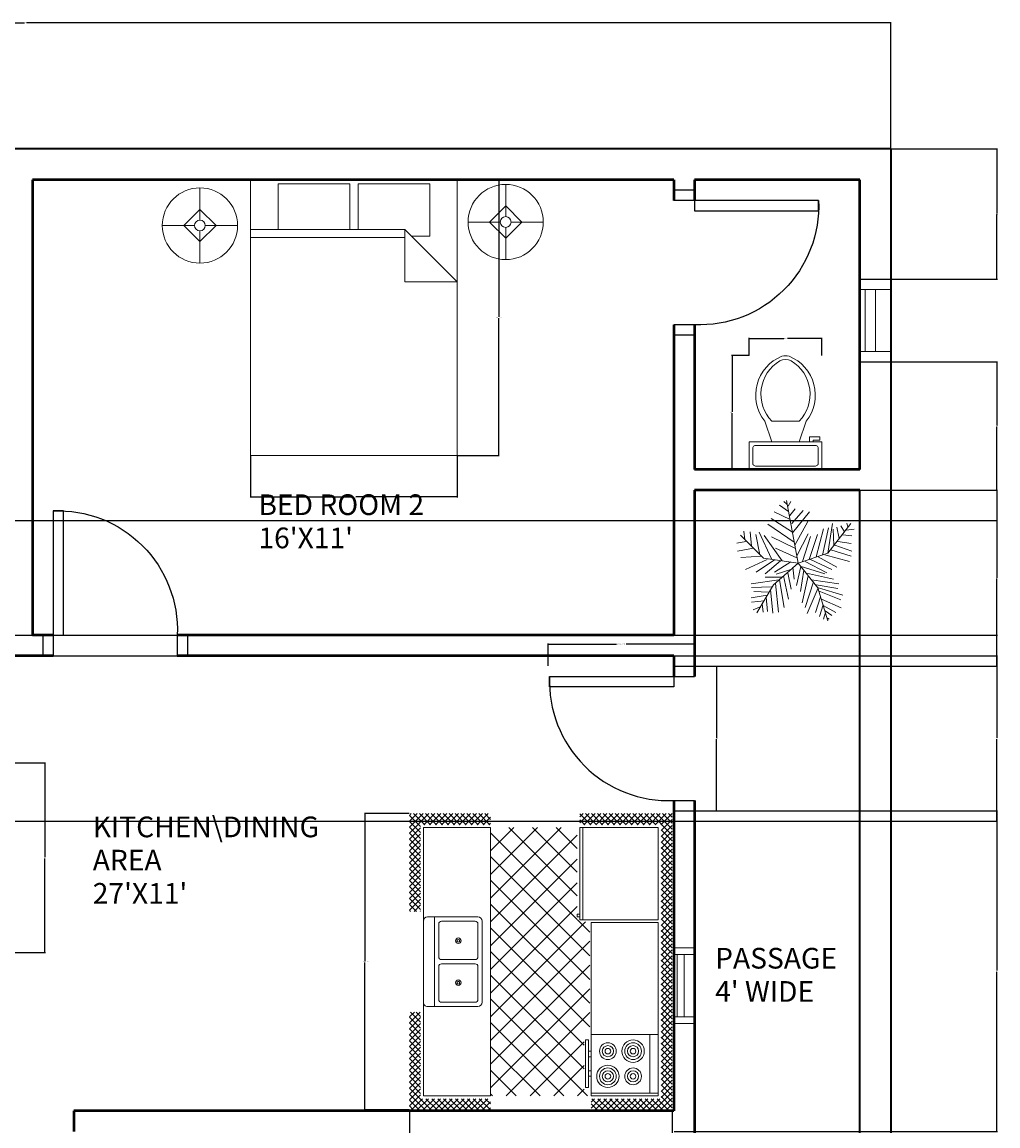
# Model space of a CAD drawing. Units: inches. Extents: x 156 to 720, y 11 to 679.
# Tile 5 of 5: x 437 to 720, y 359 to 679. Entities that reach past the tile are written whole.
import ezdxf

# ---------------------------------------------------------------- set-up
doc = ezdxf.new("R2010")
doc.units = ezdxf.units.IN
for name, color, linetype, lineweight in [('A-ANNO-DIMS', 2, 'Continuous', 18), ('A-AREA-IDEN', 7, 'Continuous', 25), ('A-DOOR', 3, 'Continuous', 25), ('A-FLOR-FIXT', 9, 'Continuous', 18), ('A-FURN', 8, 'Continuous', 18), ('A-GLAZ', 4, 'Continuous', 18), ('A-WALL', 7, 'Continuous', 50), ('C-PROP', 7, 'Continuous', 35), ('E-LITE', 2, 'Continuous', 13), ('L-PLNT', 94, 'Continuous', 13)]:
    doc.layers.add(name, color=color, linetype=linetype, lineweight=lineweight)
doc.styles.get("Standard").update_dxf_attribs({"font": 'arial.ttf'})
doc.dimstyles.get("Standard").update_dxf_attribs({"dimtxt": 0.18, "dimasz": 0.18, "dimexe": 0.18, "dimexo": 0.0625, "dimgap": 0.09, "dimtad": 0, "dimtih": 1, "dimtoh": 1, "dimdec": 4, "dimzin": 0, "dimdsep": 46, "dimtxsty": 'Standard', "dimcen": 0.09, "dimadec": 0, "dimazin": 0, "dimtfac": 1, "dimtdec": 4, "dimtofl": 0, "dimtmove": 0, "dimatfit": 3, "dimfxl": 1, "dimtolj": 1, "dimtzin": 0, "dimarcsym": 0})

# ---------------------------------------------------------------- blocks, each defined once
blk = doc.blocks.new('Kitchen Layout - 7 x 8 ft')
for p, q in [((-5, 81.32), (2.68, 89)), ((-5, 83.44), (0.56, 89)), ((-5, 85.56), (-1.56, 89)), ((-5, 87.68), (-3.68, 89)), ((-1, 84.97), (-5, 88.97)), ((1.09, 85), (-2.91, 89)), ((3.21, 85), (-0.79, 89)), ((0.81, 85), (4.81, 89)), ((5.34, 85), (1.34, 89)), ((2.93, 85), (6.93, 89)), ((7.46, 85), (3.46, 89)), ((5.05, 85), (9.05, 89)), ((9.58, 85), (5.58, 89)), ((7.17, 85), (11.17, 89)), ((11.7, 85), (7.7, 89)), ((9.29, 85), (13.29, 89)), ((13.82, 85), (9.82, 89)), ((11.41, 85), (15.41, 89)), ((15.94, 85), (11.94, 89)), ((13.53, 85), (17.53, 89)), ((18.06, 85), (14.06, 89)), ((15.65, 85), (19.65, 89)), ((20.18, 85), (16.18, 89)), ((17.78, 85), (21.78, 89)), ((22.31, 85), (18.31, 89)), ((19.9, 85), (23.9, 89)), ((24.43, 85), (20.43, 89)), ((22.02, 85), (26.02, 89)), ((26.55, 85), (22.55, 89)), ((24.14, 85), (28.14, 89)), ((28.67, 85), (24.67, 89)), ((26.26, 85), (30.26, 89)), ((30.79, 85), (26.79, 89)), ((28.38, 85), (32.38, 89)), ((32.91, 85), (28.91, 89)), ((30.5, 85), (34.5, 89)), ((35.03, 85), (31.03, 89)), ((32.63, 85), (36.63, 89)), ((37.16, 85), (33.16, 89)), ((34.75, 85), (38.75, 89)), ((39.28, 85), (35.28, 89)), ((36.87, 85), (40.87, 89)), ((41.4, 85), (37.4, 89)), ((38.99, 85), (42.99, 89)), ((43.52, 85), (39.52, 89)), ((41.11, 85), (45.11, 89)), ((45.64, 85), (41.64, 89)), ((43.23, 85), (47.23, 89)), ((47.76, 85), (43.76, 89)), ((45.35, 85), (49.35, 89)), ((49.88, 85), (45.88, 89)), ((47.47, 85), (51.47, 89)), ((52, 85), (48, 89)), ((49.6, 85), (53.6, 89)), ((54.13, 85), (50.13, 89)), ((51.72, 85), (55.72, 89)), ((56.25, 85), (52.25, 89)), ((53.84, 85), (57.84, 89)), ((58.37, 85), (54.37, 89)), ((55.96, 85), (59.96, 89)), ((60.49, 85), (56.49, 89)), ((58.08, 85), (62.08, 89)), ((62.61, 85), (58.61, 89)), ((60.2, 85), (64.2, 89)), ((64.73, 85), (60.73, 89)), ((62.32, 85), (66.32, 89)), ((66.85, 85), (62.85, 89)), ((64.45, 85), (68.45, 89)), ((68.97, 85), (64.97, 89)), ((66.57, 85), (70.57, 89)), ((71.1, 85), (67.1, 89)), ((68.69, 85), (72.69, 89)), ((73.22, 85), (69.22, 89)), ((70.81, 85), (74.81, 89)), ((75.34, 85), (71.34, 89)), ((72.93, 85), (76.93, 89)), ((77.46, 85), (73.46, 89)), ((75.05, 85), (79.05, 89)), ((79.58, 85), (75.58, 89)), ((77.17, 85), (81.17, 89)), ((81.7, 85), (77.7, 89)), ((79.29, 85), (83.29, 89)), ((83.82, 85), (79.82, 89)), ((81.42, 85), (85.42, 89)), ((85.95, 85), (81.95, 89)), ((83.54, 85), (87.54, 89)), ((88.07, 85), (84.07, 89)), ((85.66, 85), (89.66, 89)), ((90.19, 85), (86.19, 89)), ((87.78, 85), (91.78, 89)), ((92.31, 85), (88.31, 89)), ((89.9, 85), (93.9, 89)), ((94.43, 85), (90.43, 89)), ((92.02, 85), (96.02, 89)), ((96.55, 85), (92.55, 89)), ((94.14, 85), (98.14, 89)), ((101, 82.67), (94.67, 89)), ((96.27, 85), (100.27, 89)), ((101, 84.79), (96.79, 89)), ((97, 83.61), (101, 87.61)), ((101, 86.92), (98.92, 89)), ((-1, 82.85), (-5, 86.85)), ((-1, 80.73), (-5, 84.73)), ((-5, 79.19), (-1, 83.19)), ((34, 84), (96, 84)), ((34, 60), (34, 84)), ((96, 84), (96, 60)), ((97, 81.49), (101, 85.49)), ((101, 80.55), (97, 84.55)), ((97, 79.37), (101, 83.37)), ((-1, 78.61), (-5, 82.61)), ((-5, 77.07), (-1, 81.07)), ((-1, 76.49), (-5, 80.49)), ((74, 81), (95, 81)), ((101, 78.43), (97, 82.43)), ((97, 77.25), (101, 81.25)), ((101, 76.31), (97, 80.31)), ((97, 75.13), (101, 79.13)), ((-5, 74.95), (-1, 78.95)), ((-1, 74.36), (-5, 78.36)), ((-5, 72.83), (-1, 76.83)), ((-1, 72.24), (-5, 76.24)), ((101, 74.19), (97, 78.19)), ((97, 73.01), (101, 77.01)), ((101, 72.07), (97, 76.07)), ((-5, 70.71), (-1, 74.71)), ((-1, 70.12), (-5, 74.12)), ((-5, 68.59), (-1, 72.59)), ((-1, 68), (-5, 72)), ((97, 70.89), (101, 74.89)), ((101, 69.95), (97, 73.95)), ((97, 68.76), (101, 72.76)), ((101, 67.82), (97, 71.82)), ((-5, 66.47), (-1, 70.47)), ((-1, 65.88), (-5, 69.88)), ((-5, 64.35), (-1, 68.35)), ((-1, 63.76), (-5, 67.76)), ((97, 66.64), (101, 70.64)), ((101, 65.7), (97, 69.7)), ((97, 64.52), (101, 68.52)), ((101, 63.58), (97, 67.58)), ((-5, 62.22), (-1, 66.22)), ((-1, 61.64), (-5, 65.64)), ((-5, 60.1), (-1, 64.1)), ((-1, 59.52), (-5, 63.52)), ((97, 62.4), (101, 66.4)), ((101, 61.46), (97, 65.46)), ((97, 60.28), (101, 64.28)), ((100.34, 60), (97, 63.34)), ((-5, 57.98), (-1, 61.98)), ((-1, 57.39), (-5, 61.39)), ((-1.73, 56), (-5, 59.27)), ((-4.86, 56), (-1, 59.86)), ((10.4, 24), (45.9, 59.5)), ((18.88, 24), (54.38, 59.5)), ((27.37, 24), (62.87, 59.5)), ((33.03, 55.11), (37.41, 59.5)), ((96, 60), (34, 60)), ((35.85, 24), (71.35, 59.5)), ((76.2, 24), (40.7, 59.5)), ((84.68, 24), (49.18, 59.5)), ((93.17, 24), (57.67, 59.5)), ((96, 29.65), (66.15, 59.5)), ((80, 60), (80, 59)), ((82, 59), (82, 60)), ((87, 59), (87, 60)), ((89, 60), (89, 59)), ((98.22, 60), (97, 61.22)), ((98.84, 60), (101, 62.16)), ((100.96, 60), (101, 60.04)), ((-3.85, 56), (-5, 57.15)), ((-2.74, 56), (-1, 57.74)), ((0, 57), (33, 57)), ((31, 55), (31, 56)), ((32, 56), (32, 55)), ((67.71, 24), (33.68, 58.04)), ((44.34, 24), (77.84, 57.5)), ((52.82, 24), (86.32, 57.5)), ((61.31, 24), (96, 58.69)), ((96, 38.14), (76.64, 57.5)), ((96, 46.63), (85.13, 57.5)), ((96, 55.11), (93.57, 57.54)), ((0, 30.57), (24.43, 55)), ((0, 39.06), (15.94, 55)), ((0, 47.54), (7.46, 55)), ((1.91, 24), (32.91, 55)), ((33.77, 24), (2.77, 55)), ((42.26, 24), (11.26, 55)), ((50.74, 24), (19.74, 55)), ((59.23, 24), (28.23, 55)), ((32, 55), (31, 55)), ((25.29, 24), (0, 49.29)), ((69.79, 24), (96, 50.21)), ((16.8, 24), (0, 40.8)), ((78.28, 24), (96, 41.72)), ((8.32, 24), (0, 32.32)), ((86.76, 24), (96, 33.24)), ((-5, 21.92), (-2.92, 24)), ((-5, 19.8), (-1, 23.8)), ((-1, 21.33), (-3.67, 24)), ((-1, 23.45), (-1.55, 24)), ((0, 24), (96, 24)), ((0, 0), (0, 24)), ((95.25, 24), (96, 24.75)), ((96, 24), (96, 0)), ((97, 22.1), (98.9, 24)), ((97, 19.97), (101, 23.97)), ((101, 21.16), (98.16, 24)), ((101, 23.28), (100.28, 24)), ((-1, 19.21), (-5, 23.21)), ((-5, 17.68), (-1, 21.68)), ((-1, 17.09), (-5, 21.09)), ((101, 19.03), (97, 23.03)), ((97, 17.85), (101, 21.85)), ((101, 16.91), (97, 20.91)), ((-5, 15.55), (-1, 19.55)), ((-1, 14.97), (-5, 18.97)), ((-5, 13.43), (-1, 17.43)), ((-1, 12.85), (-5, 16.85)), ((47.25, 6.5), (47.25, 18.5)), ((48.75, 18.5), (48.75, 6.5)), ((97, 15.73), (101, 19.73)), ((101, 14.79), (97, 18.79)), ((97, 13.61), (101, 17.61)), ((101, 12.67), (97, 16.67)), ((-5, 11.31), (-1, 15.31)), ((-1, 10.73), (-5, 14.73)), ((-5, 9.19), (-1, 13.19)), ((-1, 8.6), (-5, 12.6)), ((97, 11.49), (101, 15.49)), ((101, 10.55), (97, 14.55)), ((97, 9.37), (101, 13.37)), ((101, 8.43), (97, 12.43)), ((-5, 7.07), (-1, 11.07)), ((-1, 6.48), (-5, 10.48)), ((-5, 4.95), (-1, 8.95)), ((-1, 4.36), (-5, 8.36)), ((97, 7.25), (101, 11.25)), ((101, 6.31), (97, 10.31)), ((97, 5.12), (101, 9.12)), ((101, 4.18), (97, 8.18)), ((-5, 2.83), (-1, 6.83)), ((-1, 2.24), (-5, 6.24)), ((-5, 0.71), (-1, 4.71)), ((-1, 0.12), (-5, 4.12)), ((64, 4), (32, 4)), ((97, 3), (101, 7)), ((101, 2.06), (97, 6.06)), ((97, 0.88), (101, 4.88)), ((-5, -1.42), (-1, 2.58)), ((2, -5), (-5, 2)), ((-5, -3.54), (-1, 0.46)), ((96, 0), (0, 0)), ((93.24, -5), (101, 2.76)), ((95.36, -5), (101, 0.64)), ((101, -0.06), (97, 3.94)), ((101, -2.18), (97, 1.82)), ((-0.12, -5), (-5, -0.12)), ((-2.25, -5), (-5, -2.25)), ((-4.34, -5), (-0.34, -1)), ((-2.22, -5), (1.78, -1)), ((-0.1, -5), (3.9, -1)), ((4.12, -5), (0.12, -1)), ((2.02, -5), (6.02, -1)), ((6.24, -5), (2.24, -1)), ((4.14, -5), (8.14, -1)), ((8.36, -5), (4.36, -1)), ((6.27, -5), (10.27, -1)), ((10.48, -5), (6.48, -1)), ((8.39, -5), (12.39, -1)), ((12.6, -5), (8.6, -1)), ((10.51, -5), (14.51, -1)), ((14.73, -5), (10.73, -1)), ((12.63, -5), (16.63, -1)), ((16.85, -5), (12.85, -1)), ((14.75, -5), (18.75, -1)), ((18.97, -5), (14.97, -1)), ((16.87, -5), (20.87, -1)), ((21.09, -5), (17.09, -1)), ((18.99, -5), (22.99, -1)), ((23.21, -5), (19.21, -1)), ((21.11, -5), (25.11, -1)), ((25.33, -5), (21.33, -1)), ((23.24, -5), (27.24, -1)), ((27.45, -5), (23.45, -1)), ((25.36, -5), (29.36, -1)), ((29.57, -5), (25.57, -1)), ((27.48, -5), (30, -2.48)), ((30, -3.3), (27.7, -1)), ((30, -1.18), (29.82, -1)), ((66, -2.54), (67.54, -1)), ((66, -4.66), (69.66, -1)), ((69.88, -5), (66, -1.12)), ((67.76, -5), (66, -3.24)), ((67.78, -5), (71.78, -1)), ((72, -5), (68, -1)), ((69.9, -5), (73.9, -1)), ((74.12, -5), (70.12, -1)), ((72.03, -5), (76.03, -1)), ((76.24, -5), (72.24, -1)), ((74.15, -5), (78.15, -1)), ((78.36, -5), (74.36, -1)), ((76.27, -5), (80.27, -1)), ((80.49, -5), (76.49, -1)), ((78.39, -5), (82.39, -1)), ((82.61, -5), (78.61, -1)), ((80.51, -5), (84.51, -1)), ((84.73, -5), (80.73, -1)), ((82.63, -5), (86.63, -1)), ((86.85, -5), (82.85, -1)), ((84.75, -5), (88.75, -1)), ((88.97, -5), (84.97, -1)), ((86.88, -5), (90.88, -1)), ((91.09, -5), (87.09, -1)), ((89, -5), (93, -1)), ((93.21, -5), (89.21, -1)), ((91.12, -5), (95.12, -1)), ((95.34, -5), (91.34, -1)), ((97.46, -5), (93.46, -1)), ((99.58, -5), (95.58, -1)), ((101, -4.3), (97, -0.3)), ((97.48, -5), (101, -1.48)), ((99.6, -5), (101, -3.6)), ((-4.37, -5), (-5, -4.37)), ((29.6, -5), (30, -4.6))]:
    blk.add_line(p, q)
for points in [[(0, 56), (0, 84), (33, 84), (33, 56)], [(74, 60), (74, 84), (95, 84), (95, 60)], [(76, 58), (76, 59), (93, 59), (93, 58)]]:
    blk.add_lwpolyline(points, close=True)
for points in [[(33.5, 21), (62.5, 21)], [(32, 1.5), (32, 19.5)], [(33.5, 6.5), (33.5, 18.5)], [(34.5, 19.5), (46.25, 19.5)], [(49.75, 19.5), (61.5, 19.5)], [(62.5, 18.5), (62.5, 6.5)], [(64, 19.5), (64, 1.5)], [(46.25, 5.5), (34.5, 5.5)], [(61.5, 5.5), (49.75, 5.5)], [(62.5, 0), (33.5, 0)]]:
    blk.add_lwpolyline(points)
for centre, radius in [((80, 75), 4), ((80, 75), 3), ((80, 75), 2), ((80, 75), 1), ((89, 75), 3), ((89, 75), 2), ((89, 75), 1), ((80, 66), 3), ((80, 66), 2), ((89, 66), 4), ((89, 66), 3), ((89, 66), 2), ((80, 66), 1), ((89, 66), 1), ((40.5, 12.5), 1), ((40.5, 12.5), 0.5), ((55.5, 12.5), 1), ((55.5, 12.5), 0.5)]:
    blk.add_circle(centre, radius)
for centre, radius, start, end in [((33.5, 19.5), 1.5, 90, 180), ((62.5, 19.5), 1.5, 0, 90), ((34.5, 18.5), 1, 90, 180), ((46.25, 18.5), 1, 0, 90), ((49.75, 18.5), 1, 90, 180), ((61.5, 18.5), 1, 0, 90), ((34.5, 6.5), 1, 180, 270), ((46.25, 6.5), 1, 270, 0), ((49.75, 6.5), 1, 180, 270), ((61.5, 6.5), 1, 270, 0), ((33.5, 1.5), 1.5, 180, 270), ((62.5, 1.5), 1.5, 270, 0)]:
    blk.add_arc(centre, radius, start, end)
blk = doc.blocks.new('Bed - Queen')
for p, q in [((0, -80.00003), (0, 0)), ((0, 0), (59.99999, 0)), ((59.99999, 0), (59.99999, -80.00003)), ((7.99999, -1.2), (28.79998, -1.2)), ((7.99999, -14.4), (7.99999, -1.2)), ((28.79998, -1.2), (28.79998, -14.4)), ((31.19999, -1.2), (51.99999, -1.2)), ((31.19999, -14.4), (31.19999, -1.2)), ((51.99999, -1.2), (51.99999, -16.4)), ((0, -14.4), (44.8, -14.4)), ((59.99999, -29.6), (44.8, -14.4)), ((44.8, -14.4), (44.8, -29.6)), ((44.8, -16.8), (0, -16.8)), ((51.99999, -16.4), (46.79936, -16.4)), ((44.8, -29.6), (59.99999, -29.6)), ((59.99999, -80.00003), (0, -80.00003))]:
    blk.add_line(p, q)
blk = doc.blocks.new('Lamp - Table')
for p, q in [((0, 7), (0, 1)), ((0, 3), (-3, 0)), ((3, 0), (0, 3)), ((-1, 0), (-7, 0)), ((-3, 0), (0, -3)), ((0, -3), (3, 0)), ((1, 0), (7, 0)), ((0, -1), (0, -7))]:
    blk.add_line(p, q)
for radius in [7, 1]:
    blk.add_circle((0, 0), radius)
blk = doc.blocks.new('*U13')
for p, q in [((-8.737, 47.138), (-17.069, 52.711)), ((-10.186, 53.64), (-13.084, 55.962)), ((0, 0), (-10.5, 57)), ((-9.099, 51.782), (-6.563, 55.962)), ((-5.114, 28.097), (-24.676, 40.636)), ((-7.288, 39.707), (-21.778, 46.673)), ((-7.65, 43.423), (-2.578, 49.46)), ((-5.839, 35.992), (4.667, 48.067)), ((-5.114, 27.632), (10.463, 46.673)), ((-3.665, 19.273), (-27.574, 35.527)), ((-2.941, 16.486), (8.652, 37.85)), ((16.259, 5.805), (23.142, 31.348)), ((22.055, 7.198), (27.489, 32.277)), ((27, 9), (48, 36)), ((27.127, 9.056), (31.112, 35.992)), ((31.836, 30.883), (32.561, 16.486)), ((35.096, 32.741), (37.27, 22.524)), ((38.719, 34.134), (41.979, 28.561)), ((43.791, 29.954), (51.036, 30.883)), ((44.153, 36.456), (45.239, 32.741)), ((-31.5, 4.5), (-52.5, 25.5)), ((-48.585, 21.131), (-49.309, 29.026)), ((-43.513, 28.561), (-42.427, 15.558)), ((-38.442, 26.239), (-34.819, 7.663)), ((-35.544, 28.097), (-24.314, 3.947)), ((-14.533, 2.09), (-30.834, 25.31)), ((-24.314, 23.917), (-2.941, 13.7)), ((-1.129, 6.734), (9.014, 26.704)), ((3.942, 1.625), (11.187, 24.381)), ((10.101, 3.483), (17.708, 26.239)), ((40.53, 25.775), (48.862, 24.846)), ((-47.498, 19.737), (-55.83, 18.344)), ((-40.615, 13.7), (-55.105, 10.913)), ((-20.691, 13.7), (-1.129, 4.876)), ((29.662, 12.307), (48.137, 6.269)), ((33.285, 16.486), (48.862, 10.913)), ((36.183, 19.737), (48.137, 17.88)), ((-33.37, 6.269), (-52.207, 5.34)), ((-28.299, 3.483), (-47.86, -5.805)), ((-21.416, 3.018), (-38.079, -8.128)), ((0, 0), (-31.5, 4.5)), ((-15.982, 2.09), (-30.11, -9.521)), ((0, 0), (-22.5, -19.5)), ((-6.563, 1.161), (-21.416, -8.128)), ((0, 0), (27, 9)), ((0, 0), (18, -22.5)), ((6.478, 1.625), (26.04, -8.592)), ((11.187, 3.483), (30.749, -5.805)), ((18.07, 5.805), (35.096, -3.483)), ((24.229, 7.663), (46.688, 1.625)), ((-6.563, -5.805), (-19.967, -9.985)), ((-9.461, -8.592), (-6.201, -23.453)), ((-4.752, -3.483), (-3.665, -14.629)), ((2.493, -3.019), (-1.491, -20.202)), ((1.769, -2.555), (24.229, -9.521)), ((5.029, -6.27), (2.131, -25.775)), ((7.565, -9.056), (32.198, -14.629)), ((-17.431, -15.094), (-42.789, -18.809)), ((-22.5, -19.5), (-37.5, -45)), ((-15.257, -12.772), (-30.11, -12.772)), ((-20.691, -18.345), (-17.793, -44.352)), ((-17.069, -15.094), (-12.721, -40.172)), ((-13.446, -11.378), (-8.737, -32.741)), ((9.014, -11.378), (3.58, -35.992)), ((14.085, -16.951), (6.478, -40.172)), ((12.274, -15.094), (36.907, -18.809)), ((16.259, -19.738), (36.183, -22.989)), ((-28.299, -29.026), (-42.789, -31.348)), ((-24.314, -21.596), (-42.427, -22.06)), ((-26.849, -26.24), (-40.253, -25.775)), ((-25.038, -23.918), (-22.865, -45.281)), ((18.07, -22.524), (8.289, -45.745)), ((18, -22.5), (27, -52.5)), ((18.433, -22.524), (40.53, -29.026)), ((19.157, -25.311), (38.719, -33.206)), ((-30.834, -34.135), (-42.427, -35.528)), ((-34.457, -39.708), (-40.978, -42.494)), ((-32.646, -36.921), (-31.921, -44.352)), ((-29.023, -30.884), (-27.936, -43.887)), ((20.244, -30.419), (15.897, -44.816)), ((22.78, -37.85), (19.519, -48.532)), ((21.331, -32.741), (39.081, -40.636)), ((22.78, -38.314), (34.372, -44.816)), ((24.591, -45.745), (23.142, -50.854)), ((24.591, -43.423), (30.749, -47.603)), ((26.764, -49.925), (28.213, -50.854))]:
    blk.add_line(p, q)
blk = doc.blocks.new('Toilet - top')
for p, q in [((9.5, -6), (9.5, -2)), ((-10, -8.5), (-8, -8.5)), ((-10, -9.5), (-10, -8.5)), ((-7, -9.5), (-10, -9.5)), ((-8, -8.5), (-8, -8)), ((-7, -8), (-7, -9.5)), ((-4, -8), (-6, -14)), ((4, -8), (6, -14)), ((4, -14), (-4, -14))]:
    blk.add_line(p, q)
blk.add_lwpolyline([(10.5, -8), (10.5, 0), (-10.5, 0), (-10.5, -8)], close=True)
for points in [[(-9.5, -2), (-9.5, -6)], [(8.5, -1), (-8.5, -1)], [(-8.5, -7), (8.5, -7)]]:
    blk.add_lwpolyline(points)
for centre, radius, start, end in [((-8.62, -1.88), 0.884, 81.8699, 188.1301), ((8.62, -1.88), 0.884, 351.8699, 98.1301), ((-8.62, -6.12), 0.884, 171.8699, 278.1301), ((8.62, -6.12), 0.884, 261.8699, 8.1301), ((3.52, -21.58), 12.17, 141.4691, 247.9714), ((4.2, -21.82), 11.33, 136.3677, 238.9468), ((-3.52, -21.58), 12.17, 292.0284, 38.5307), ((-4.2, -21.82), 11.33, 301.053, 43.6321), ((0, -27.88), 4, 245.7318, 294.2682), ((0, -29), 4, 254.8605, 285.1395)]:
    blk.add_arc(centre, radius, start, end)
blk = doc.blocks.new('DOOR-SWING-36IN')
for p, q in [((0, 6), (0, 0)), ((3, 6), (3, 0)), ((39, 6), (39, 0)), ((42, 6), (42, 0))]:
    blk.add_line(p, q)
blk.add_lwpolyline([(39, 6), (36, 6), (36, 42), (39, 42)], close=True)
blk.add_arc((37.5, 7.5), 34.53, 87.5104, 182.4896)
blk = doc.blocks.new('WIN-18IN-WALL9')
for p, q in [((9, 24), (0, 24)), ((0, 21), (0, 3)), ((9, 21), (0, 21)), ((4.5, 21), (4.5, 3)), ((7.5, 21), (7.5, 3)), ((9, 3), (9, 21)), ((0, 3), (9, 3)), ((0, 0), (9, 0))]:
    blk.add_line(p, q)
blk = doc.blocks.new('*D21')
at = {"layer": 'A-ANNO-DIMS', "color": 0, "lineweight": -2, "transparency": 16777216}
for p, q in [((589.3, 492.21), (589.3, 498.69)), ((589.48, 498.51), (609.11, 498.51)), ((631.54, 498.51), (611.91, 498.51)), ((631.72, 492.21), (631.72, 498.69))]:
    blk.add_line(p, q, dxfattribs=at)
at = {"layer": 'A-ANNO-DIMS', "color": 0, "transparency": 16777216}
for points in [[(589.48, 498.54), (589.48, 498.48), (589.3, 498.51)], [(631.54, 498.54), (631.54, 498.48), (631.72, 498.51)]]:
    blk.add_solid(points, dxfattribs=at)
at = {"layer": 'Defpoints', "color": 0, "transparency": 16777216}
for p in [(589.3, 498.51), (589.3, 492.15), (631.72, 492.15)]:
    blk.add_point(p, dxfattribs=at)
at = {"layer": 'A-ANNO-DIMS', "color": 0, "transparency": 16777216, "insert": (610.51, 498.51), "char_height": 0.18, "attachment_point": 5}
blk.add_mtext('\\A1;SWING DOOR 42 TYP.', dxfattribs=at)
blk = doc.blocks.new('*D22')
at = {"layer": 'A-ANNO-DIMS', "color": 0, "lineweight": -2, "transparency": 16777216}
for p, q in [((631.79, 492.15), (638.27, 492.15)), ((638.09, 491.97), (638.09, 471.33)), ((638.09, 450.33), (638.09, 470.97)), ((631.79, 450.15), (638.27, 450.15))]:
    blk.add_line(p, q, dxfattribs=at)
at = {"layer": 'A-ANNO-DIMS', "color": 0, "transparency": 16777216}
for points in [[(638.06, 491.97), (638.12, 491.97), (638.09, 492.15)], [(638.06, 450.33), (638.12, 450.33), (638.09, 450.15)]]:
    blk.add_solid(points, dxfattribs=at)
at = {"layer": 'Defpoints', "color": 0, "transparency": 16777216}
for p in [(631.72, 492.15), (638.09, 492.15), (631.72, 450.15)]:
    blk.add_point(p, dxfattribs=at)
at = {"layer": 'A-ANNO-DIMS', "color": 0, "transparency": 16777216, "insert": (638.09, 471.15), "char_height": 0.18, "attachment_point": 5}
blk.add_mtext('\\A1;42 TYP.', dxfattribs=at)
blk = doc.blocks.new('*D25')
at = {"layer": 'A-ANNO-DIMS', "color": 0, "lineweight": -2, "transparency": 16777216}
for p, q in [((563.01, 633.21), (575.13, 633.21)), ((574.95, 633.03), (574.95, 593.4)), ((574.95, 553.39), (574.95, 593.02)), ((563.01, 553.21), (575.13, 553.21))]:
    blk.add_line(p, q, dxfattribs=at)
at = {"layer": 'A-ANNO-DIMS', "color": 0, "transparency": 16777216}
for points in [[(574.92, 633.03), (574.98, 633.03), (574.95, 633.21)], [(574.92, 553.39), (574.98, 553.39), (574.95, 553.21)]]:
    blk.add_solid(points, dxfattribs=at)
at = {"layer": 'Defpoints', "color": 0, "transparency": 16777216}
for p in [(562.95, 633.21), (574.95, 633.21), (562.95, 553.21)]:
    blk.add_point(p, dxfattribs=at)
at = {"layer": 'A-ANNO-DIMS', "color": 0, "transparency": 16777216, "insert": (574.95, 593.21), "char_height": 0.18, "attachment_point": 5}
blk.add_mtext('\\A1;QUEEN BED 80 TYP.', dxfattribs=at)
blk = doc.blocks.new('*D26')
at = {"layer": 'A-ANNO-DIMS', "color": 0, "lineweight": -2, "transparency": 16777216}
for p, q in [((502.95, 553.15), (502.95, 541.03)), ((562.95, 553.15), (562.95, 541.03)), ((503.13, 541.21), (532.42, 541.21)), ((562.77, 541.21), (533.47, 541.21))]:
    blk.add_line(p, q, dxfattribs=at)
at = {"layer": 'A-ANNO-DIMS', "color": 0, "transparency": 16777216}
for points in [[(503.13, 541.24), (503.13, 541.18), (502.95, 541.21)], [(562.77, 541.24), (562.77, 541.18), (562.95, 541.21)]]:
    blk.add_solid(points, dxfattribs=at)
at = {"layer": 'Defpoints', "color": 0, "transparency": 16777216}
for p in [(502.95, 553.21), (562.95, 553.21), (562.95, 541.21)]:
    blk.add_point(p, dxfattribs=at)
at = {"layer": 'A-ANNO-DIMS', "color": 0, "transparency": 16777216, "insert": (532.95, 541.21), "char_height": 0.18, "attachment_point": 5}
blk.add_mtext('\\A1;60 TYP.', dxfattribs=at)
blk = doc.blocks.new('*D27')
at = {"layer": 'A-ANNO-DIMS', "color": 0, "lineweight": -2, "transparency": 16777216}
for p, q in [((647.56, 582.2), (642.49, 582.2)), ((642.67, 582.02), (642.67, 565.86)), ((642.67, 549.33), (642.67, 565.49)), ((647.56, 549.15), (642.49, 549.15))]:
    blk.add_line(p, q, dxfattribs=at)
at = {"layer": 'A-ANNO-DIMS', "color": 0, "transparency": 16777216}
for points in [[(642.64, 582.02), (642.7, 582.02), (642.67, 582.2)], [(642.64, 549.33), (642.7, 549.33), (642.67, 549.15)]]:
    blk.add_solid(points, dxfattribs=at)
at = {"layer": 'Defpoints', "color": 0, "transparency": 16777216}
for p in [(647.63, 582.2), (642.67, 549.15), (647.63, 549.15)]:
    blk.add_point(p, dxfattribs=at)
at = {"layer": 'A-ANNO-DIMS', "color": 0, "transparency": 16777216, "insert": (642.67, 565.67), "char_height": 0.18, "attachment_point": 5}
blk.add_mtext('\\A1;WC 33 TYP.', dxfattribs=at)
blk = doc.blocks.new('*D28')
at = {"layer": 'A-ANNO-DIMS', "color": 0, "lineweight": -2, "transparency": 16777216}
for p, q in [((647.63, 582.26), (647.63, 587.33)), ((647.81, 587.15), (657.6, 587.15)), ((668.45, 587.15), (658.66, 587.15)), ((668.63, 582.26), (668.63, 587.33))]:
    blk.add_line(p, q, dxfattribs=at)
at = {"layer": 'A-ANNO-DIMS', "color": 0, "transparency": 16777216}
for points in [[(647.81, 587.18), (647.81, 587.12), (647.63, 587.15)], [(668.45, 587.18), (668.45, 587.12), (668.63, 587.15)]]:
    blk.add_solid(points, dxfattribs=at)
at = {"layer": 'Defpoints', "color": 0, "transparency": 16777216}
for p in [(647.63, 587.15), (647.63, 582.2), (668.63, 582.2)]:
    blk.add_point(p, dxfattribs=at)
at = {"layer": 'A-ANNO-DIMS', "color": 0, "transparency": 16777216, "insert": (658.13, 587.15), "char_height": 0.18, "attachment_point": 5}
blk.add_mtext('\\A1;21 TYP.', dxfattribs=at)
blk = doc.blocks.new('*D37')
at = {"layer": 'A-ANNO-DIMS', "color": 0, "lineweight": -2, "transparency": 16777216}
for p, q in [((548.99, 449.36), (535.99, 449.36)), ((536.17, 449.18), (536.17, 406.58)), ((536.17, 363.6), (536.17, 406.21)), ((548.99, 363.42), (535.99, 363.42))]:
    blk.add_line(p, q, dxfattribs=at)
at = {"layer": 'A-ANNO-DIMS', "color": 0, "transparency": 16777216}
for points in [[(536.14, 449.18), (536.2, 449.18), (536.17, 449.36)], [(536.14, 363.6), (536.2, 363.6), (536.17, 363.42)]]:
    blk.add_solid(points, dxfattribs=at)
at = {"layer": 'Defpoints', "color": 0, "transparency": 16777216}
for p in [(549.06, 449.36), (536.17, 363.42), (549.06, 363.42)]:
    blk.add_point(p, dxfattribs=at)
at = {"layer": 'A-ANNO-DIMS', "color": 0, "transparency": 16777216, "insert": (536.17, 406.39), "char_height": 0.18, "attachment_point": 5}
blk.add_mtext('\\A1;KITCHEN UNIT 86', dxfattribs=at)
blk = doc.blocks.new('*D38')
at = {"layer": 'A-ANNO-DIMS', "color": 0, "lineweight": -2, "transparency": 16777216}
for p, q in [((549.06, 363.36), (549.06, 350.35)), ((625.27, 363.36), (625.27, 350.35)), ((549.24, 350.53), (586.94, 350.53)), ((625.09, 350.53), (587.38, 350.53))]:
    blk.add_line(p, q, dxfattribs=at)
at = {"layer": 'A-ANNO-DIMS', "color": 0, "transparency": 16777216}
for points in [[(549.24, 350.56), (549.24, 350.5), (549.06, 350.53)], [(625.09, 350.56), (625.09, 350.5), (625.27, 350.53)]]:
    blk.add_solid(points, dxfattribs=at)
at = {"layer": 'Defpoints', "color": 0, "transparency": 16777216}
for p in [(549.06, 363.42), (625.27, 363.42), (625.27, 350.53)]:
    blk.add_point(p, dxfattribs=at)
at = {"layer": 'A-ANNO-DIMS', "color": 0, "transparency": 16777216, "insert": (587.16, 350.53), "char_height": 0.18, "attachment_point": 5}
blk.add_mtext('\\A1;76', dxfattribs=at)
blk = doc.blocks.new('*D42')
at = {"layer": 'A-ANNO-DIMS', "color": 0, "lineweight": -2, "transparency": 16777216}
for p, q in [((429.7, 464.06), (443.47, 464.06)), ((443.29, 463.88), (443.29, 436.74)), ((443.29, 409.24), (443.29, 436.37)), ((429.7, 409.06), (443.47, 409.06))]:
    blk.add_line(p, q, dxfattribs=at)
at = {"layer": 'A-ANNO-DIMS', "color": 0, "transparency": 16777216}
for points in [[(443.26, 463.88), (443.32, 463.88), (443.29, 464.06)], [(443.26, 409.24), (443.32, 409.24), (443.29, 409.06)]]:
    blk.add_solid(points, dxfattribs=at)
at = {"layer": 'Defpoints', "color": 0, "transparency": 16777216}
for p in [(429.64, 464.06), (443.29, 464.06), (429.64, 409.06)]:
    blk.add_point(p, dxfattribs=at)
at = {"layer": 'A-ANNO-DIMS', "color": 0, "transparency": 16777216, "insert": (443.29, 436.56), "char_height": 0.18, "attachment_point": 5}
blk.add_mtext('\\A1;55', dxfattribs=at)
blk = doc.blocks.new('*D49')
at = {"layer": 'A-ANNO-DIMS', "color": 0, "lineweight": -2, "transparency": 16777216}
for p, q in [((186.72, 642.21), (186.72, 678.94)), ((688.72, 642.21), (688.72, 678.94)), ((186.9, 678.76), (437.44, 678.76)), ((688.54, 678.76), (438.01, 678.76))]:
    blk.add_line(p, q, dxfattribs=at)
at = {"layer": 'A-ANNO-DIMS', "color": 0, "transparency": 16777216}
for points in [[(186.9, 678.79), (186.9, 678.73), (186.72, 678.76)], [(688.54, 678.79), (688.54, 678.73), (688.72, 678.76)]]:
    blk.add_solid(points, dxfattribs=at)
at = {"layer": 'Defpoints', "color": 0, "transparency": 16777216}
for p in [(688.72, 678.76), (186.72, 642.15), (688.72, 642.15)]:
    blk.add_point(p, dxfattribs=at)
at = {"layer": 'A-ANNO-DIMS', "color": 0, "transparency": 16777216, "insert": (437.72, 678.76), "char_height": 0.18, "attachment_point": 5}
blk.add_mtext('\\A1;502', dxfattribs=at)
blk = doc.blocks.new('*D62')
at = {"layer": 'A-ANNO-DIMS', "color": 0, "lineweight": -2, "transparency": 16777216}
for p, q in [((625.79, 450.15), (719.6, 450.15)), ((719.42, 449.97), (719.42, 403.83)), ((719.42, 357.33), (719.42, 403.47)), ((625.79, 357.15), (719.6, 357.15))]:
    blk.add_line(p, q, dxfattribs=at)
at = {"layer": 'A-ANNO-DIMS', "color": 0, "transparency": 16777216}
for points in [[(719.39, 449.97), (719.45, 449.97), (719.42, 450.15)], [(719.39, 357.33), (719.45, 357.33), (719.42, 357.15)]]:
    blk.add_solid(points, dxfattribs=at)
at = {"layer": 'Defpoints', "color": 0, "transparency": 16777216}
for p in [(625.72, 450.15), (719.42, 450.15), (625.72, 357.15)]:
    blk.add_point(p, dxfattribs=at)
at = {"layer": 'A-ANNO-DIMS', "color": 0, "transparency": 16777216, "insert": (719.42, 403.65), "char_height": 0.18, "attachment_point": 5}
blk.add_mtext('\\A1;93', dxfattribs=at)
blk = doc.blocks.new('*D63')
at = {"layer": 'A-ANNO-DIMS', "color": 0, "lineweight": -2, "transparency": 16777216}
for p, q in [((631.79, 543.15), (719.6, 543.15)), ((719.42, 542.97), (719.42, 517.83)), ((719.42, 492.33), (719.42, 517.47)), ((631.79, 492.15), (719.6, 492.15))]:
    blk.add_line(p, q, dxfattribs=at)
at = {"layer": 'A-ANNO-DIMS', "color": 0, "transparency": 16777216}
for points in [[(719.39, 542.97), (719.45, 542.97), (719.42, 543.15)], [(719.39, 492.33), (719.45, 492.33), (719.42, 492.15)]]:
    blk.add_solid(points, dxfattribs=at)
at = {"layer": 'Defpoints', "color": 0, "transparency": 16777216}
for p in [(631.72, 543.15), (719.42, 543.15), (631.72, 492.15)]:
    blk.add_point(p, dxfattribs=at)
at = {"layer": 'A-ANNO-DIMS', "color": 0, "transparency": 16777216, "insert": (719.42, 517.65), "char_height": 0.18, "attachment_point": 5}
blk.add_mtext('\\A1;51', dxfattribs=at)
blk = doc.blocks.new('*D64')
at = {"layer": 'A-ANNO-DIMS', "color": 0, "lineweight": -2, "transparency": 16777216}
for p, q in [((679.79, 580.37), (719.6, 580.37)), ((719.42, 580.19), (719.42, 561.94)), ((719.42, 543.33), (719.42, 561.58)), ((631.79, 543.15), (719.6, 543.15))]:
    blk.add_line(p, q, dxfattribs=at)
at = {"layer": 'A-ANNO-DIMS', "color": 0, "transparency": 16777216}
for points in [[(719.39, 580.19), (719.45, 580.19), (719.42, 580.37)], [(719.39, 543.33), (719.45, 543.33), (719.42, 543.15)]]:
    blk.add_solid(points, dxfattribs=at)
at = {"layer": 'Defpoints', "color": 0, "transparency": 16777216}
for p in [(679.72, 580.37), (719.42, 580.37), (631.72, 543.15)]:
    blk.add_point(p, dxfattribs=at)
at = {"layer": 'A-ANNO-DIMS', "color": 0, "transparency": 16777216, "insert": (719.42, 561.76), "char_height": 0.18, "attachment_point": 5}
blk.add_mtext('\\A1;37.22', dxfattribs=at)
blk = doc.blocks.new('*D65')
at = {"layer": 'A-ANNO-DIMS', "color": 0, "lineweight": -2, "transparency": 16777216}
for p, q in [((688.79, 642.15), (719.6, 642.15)), ((719.42, 641.97), (719.42, 623.44)), ((719.42, 604.55), (719.42, 623.08)), ((679.79, 604.37), (719.6, 604.37))]:
    blk.add_line(p, q, dxfattribs=at)
at = {"layer": 'A-ANNO-DIMS', "color": 0, "transparency": 16777216}
for points in [[(719.39, 641.97), (719.45, 641.97), (719.42, 642.15)], [(719.39, 604.55), (719.45, 604.55), (719.42, 604.37)]]:
    blk.add_solid(points, dxfattribs=at)
at = {"layer": 'Defpoints', "color": 0, "transparency": 16777216}
for p in [(688.72, 642.15), (719.42, 642.15), (679.72, 604.37)]:
    blk.add_point(p, dxfattribs=at)
at = {"layer": 'A-ANNO-DIMS', "color": 0, "transparency": 16777216, "insert": (719.42, 623.26), "char_height": 0.18, "attachment_point": 5}
blk.add_mtext('\\A1;37.78', dxfattribs=at)
blk = doc.blocks.new('*D67')
at = {"layer": 'A-ANNO-DIMS', "color": 0, "lineweight": -2, "transparency": 16777216}
for p, q in [((325.79, 495.15), (719.6, 495.15)), ((719.42, 494.97), (719.42, 471.33)), ((719.42, 447.33), (719.42, 470.97)), ((325.79, 447.15), (719.6, 447.15))]:
    blk.add_line(p, q, dxfattribs=at)
at = {"layer": 'A-ANNO-DIMS', "color": 0, "transparency": 16777216}
for points in [[(719.39, 494.97), (719.45, 494.97), (719.42, 495.15)], [(719.39, 447.33), (719.45, 447.33), (719.42, 447.15)]]:
    blk.add_solid(points, dxfattribs=at)
at = {"layer": 'Defpoints', "color": 0, "transparency": 16777216}
for p in [(325.72, 495.15), (719.42, 495.15), (325.72, 447.15)]:
    blk.add_point(p, dxfattribs=at)
at = {"layer": 'A-ANNO-DIMS', "color": 0, "transparency": 16777216, "insert": (719.42, 471.15), "char_height": 0.18, "attachment_point": 5}
blk.add_mtext('\\A1;48', dxfattribs=at)
blk = doc.blocks.new('*D72')
at = {"layer": 'A-ANNO-DIMS', "color": 0, "lineweight": -2, "transparency": 16777216}
for p, q in [((241.79, 534.4), (719.6, 534.4)), ((719.42, 534.22), (719.42, 517.96)), ((719.42, 501.33), (719.42, 517.59)), ((241.79, 501.15), (719.6, 501.15))]:
    blk.add_line(p, q, dxfattribs=at)
at = {"layer": 'A-ANNO-DIMS', "color": 0, "transparency": 16777216}
for points in [[(719.39, 534.22), (719.45, 534.22), (719.42, 534.4)], [(719.39, 501.33), (719.45, 501.33), (719.42, 501.15)]]:
    blk.add_solid(points, dxfattribs=at)
at = {"layer": 'Defpoints', "color": 0, "transparency": 16777216}
for p in [(241.72, 534.4), (719.42, 534.4), (241.72, 501.15)]:
    blk.add_point(p, dxfattribs=at)
at = {"layer": 'A-ANNO-DIMS', "color": 0, "transparency": 16777216, "insert": (719.42, 517.78), "char_height": 0.18, "attachment_point": 5}
blk.add_mtext('\\A1;33.25', dxfattribs=at)

msp = doc.modelspace()

# ---------------------------------------------------------------- linework, layer by layer
at = {"layer": 'A-GLAZ'}
for p, q in [((625.7236, 410.4548), (631.7236, 410.4548)), ((625.7236, 408.4548), (631.7236, 408.4548)), ((626.7236, 390.4548), (626.7236, 408.4548)), ((628.7236, 390.4548), (628.7236, 408.4548)), ((631.7236, 390.4548), (625.7236, 390.4548)), ((631.7236, 388.4548), (625.7236, 388.4548))]:
    msp.add_line(p, q, dxfattribs=at)
at = {"layer": 'A-WALL'}
for p, q in [((439.7236, 633.1514), (439.7236, 501.1514)), ((625.7236, 633.1514), (439.7236, 633.1514)), ((625.7236, 633.1514), (625.7236, 627.1514)), ((679.7236, 633.1514), (631.7236, 633.1514)), ((631.7236, 633.1514), (631.7236, 627.1514)), ((679.7236, 549.1514), (679.7236, 633.1514)), ((625.7236, 591.1514), (625.7236, 501.1514)), ((631.7236, 591.1514), (631.7236, 549.1514)), ((679.7236, 549.1514), (631.7236, 549.1514)), ((679.7236, 543.1514), (631.7236, 543.1514)), ((631.7236, 543.1514), (631.7236, 489.1514)), ((445.7236, 501.1514), (439.7236, 501.1514)), ((625.7236, 501.1514), (481.7236, 501.1514)), ((445.7236, 495.1514), (427.7236, 495.1514)), ((625.7236, 495.1514), (481.7236, 495.1514)), ((625.7236, 495.1514), (625.7236, 489.1514)), ((625.7236, 453.1514), (625.7236, 363.1514)), ((631.7236, 453.1514), (631.7236, 80.1514)), ((625.7236, 363.1514), (451.7236, 363.1514)), ((451.7236, 363.1514), (451.7236, 357.1514))]:
    msp.add_line(p, q, dxfattribs=at)
at = {"layer": 'C-PROP'}
for p, q in [((688.7236, 642.1514), (186.7236, 642.1514)), ((688.7236, 42.1514), (688.7236, 642.1514)), ((679.7236, 51.1514), (679.7236, 543.1514))]:
    msp.add_line(p, q, dxfattribs=at)

# ---------------------------------------------------------------- block references
at = {"layer": 'A-DOOR', "extrusion": (0, 0, -1), "zscale": -1, "rotation": 89.99999999999984}
msp.add_blockref('DOOR-SWING-36IN', (-625.7232, 588.1518), dxfattribs=at)
at = {"layer": 'A-DOOR', "extrusion": (0, 0, -1), "zscale": -1}
msp.add_blockref('DOOR-SWING-36IN', (-484.7232, 495.151), dxfattribs=at)
at = {"layer": 'A-DOOR', "rotation": 89.99999999999991}
msp.add_blockref('DOOR-SWING-36IN', (631.724, 450.1518), dxfattribs=at)
at = {"layer": 'A-FLOR-FIXT', "rotation": 180}
msp.add_blockref('Toilet - top', (658.1259, 549.1514), dxfattribs=at)
at = {"layer": 'A-FLOR-FIXT', "xscale": 0.8107505577684575, "yscale": 0.8107505577684575, "zscale": 0.8107505577684575, "rotation": 270}
msp.add_blockref('Kitchen Layout - 7 x 8 ft', (553.1104, 445.3085), dxfattribs=at)
at = {"layer": 'A-FURN'}
msp.add_blockref('Bed - Queen', (502.9454, 633.2129), dxfattribs=at)
at = {"layer": 'A-GLAZ', "rotation": 180}
msp.add_blockref('WIN-18IN-WALL9', (688.7232, 604.3678), dxfattribs=at)
at = {"layer": 'E-LITE', "xscale": 1.558829175044203, "yscale": 1.558829175044203, "zscale": 1.558829175044203}
for p in [(488.309, 619.9318), (576.9821, 620.9477)]:
    msp.add_blockref('Lamp - Table', p, dxfattribs=at)
at = {"layer": 'L-PLNT', "xscale": 0.3190560942374665, "yscale": 0.3190560942374665, "zscale": 0.3190560942374665}
msp.add_blockref('*U13', (661.7953, 521.9798), dxfattribs=at)

# ---------------------------------------------------------------- texts
at = {"layer": 'A-AREA-IDEN'}
for s, p in [('BED ROOM 2', (505.2694, 535.9558)), ("16'X11'", (505.2694, 526.3173)), ('KITCHEN\\DINING', (457.2159, 442.4974)), ('AREA', (457.2159, 432.8589)), ("27'X11'", (457.2159, 423.2205)), ('PASSAGE', (637.7216, 404.4074)), ("4' WIDE", (637.7216, 394.7689))]:
    msp.add_text(s, height=6, dxfattribs=at).set_placement(p)

# ---------------------------------------------------------------- dimensions: what is measured, and where the dimension line sits
at = {"layer": 'A-ANNO-DIMS'}
for base, p1, p2, picture, middle in [((688.7236, 678.7597), (186.7236, 642.1514), (688.7236, 642.1514), '*D49', (437.7236, 678.7597)), ((625.2672, 350.5318), (549.0567, 363.4227), (625.2672, 363.4227), '*D38', (587.1619, 350.5318))]:
    dim = msp.add_linear_dim(base=base, p1=p1, p2=p2, dimstyle='Standard', override={"dimdec": 0, "dimlfac": 1, "dimrnd": 0, "dimzin": 0, "dimdsep": 46, "dimlunit": 2}, dxfattribs=at)
    dim.commit()
    dim.dimension.update_dxf_attribs({"geometry": picture, "text_midpoint": middle})
for base, p1, p2, override, picture, middle in [((719.4236, 642.1514), (679.7236, 604.3678), (688.7236, 642.1514), {"dimdec": 2, "dimlfac": 1, "dimrnd": 0, "dimzin": 0, "dimdsep": 46, "dimlunit": 2}, '*D65', (719.4236, 623.2596)), ((719.4236, 580.3678), (631.7236, 543.1514), (679.7236, 580.3678), {"dimdec": 2, "dimlfac": 1, "dimrnd": 0, "dimzin": 0, "dimdsep": 46, "dimlunit": 2}, '*D64', (719.4236, 561.7596)), ((719.4236, 543.1514), (631.7236, 492.1514), (631.7236, 543.1514), {"dimdec": 0, "dimlfac": 1, "dimrnd": 0, "dimzin": 0, "dimdsep": 46, "dimlunit": 2}, '*D63', (719.4236, 517.6514)), ((719.4236, 534.4018), (241.7236, 501.1514), (241.7236, 534.4018), {"dimdec": 2, "dimlfac": 1, "dimrnd": 0, "dimzin": 0, "dimdsep": 46, "dimlunit": 2}, '*D72', (719.4236, 517.7766)), ((719.4236, 495.1514), (325.7236, 447.1514), (325.7236, 495.1514), {"dimdec": 0, "dimlfac": 1, "dimrnd": 0, "dimzin": 0, "dimdsep": 46, "dimlunit": 2}, '*D67', (719.4236, 471.1514)), ((443.2856, 464.056), (429.6356, 409.056), (429.6356, 464.056), {"dimdec": 0, "dimlfac": 1, "dimrnd": 0, "dimzin": 0, "dimdsep": 46, "dimlunit": 2}, '*D42', (443.2856, 436.556)), ((719.4236, 450.1514), (625.7236, 357.1514), (625.7236, 450.1514), {"dimdec": 0, "dimlfac": 1, "dimrnd": 0, "dimzin": 0, "dimdsep": 46, "dimlunit": 2}, '*D62', (719.4236, 403.6514))]:
    dim = msp.add_linear_dim(base=base, p1=p1, p2=p2, angle=90, dimstyle='Standard', override=override, dxfattribs=at)
    dim.commit()
    dim.dimension.update_dxf_attribs({"geometry": picture, "text_midpoint": middle})
for base, p1, p2, angle, text, picture, middle in [((574.9454, 633.2129), (562.9454, 553.2128), (562.9454, 633.2129), 90, 'QUEEN BED <> TYP.', '*D25', (574.9454, 593.2129)), ((647.6259, 587.1546), (668.6259, 582.1976), (647.6259, 582.1976), 180, '<> TYP.', '*D28', (658.1259, 587.1546)), ((642.669, 549.1514), (647.6259, 582.1976), (647.6259, 549.1514), 270, 'WC <> TYP.', '*D27', (642.669, 565.6745)), ((589.3031, 498.5145), (631.7236, 492.1514), (589.3031, 492.1514), 180, 'SWING DOOR <> TYP.', '*D21', (610.5134, 498.5145)), ((638.0867, 492.1514), (631.7236, 450.1514), (631.7236, 492.1514), 90, '<> TYP.', '*D22', (638.0867, 471.1514)), ((536.1657, 363.4227), (549.0567, 449.3623), (549.0567, 363.4227), 270, 'KITCHEN UNIT <>', '*D37', (536.1657, 406.3925))]:
    dim = msp.add_linear_dim(base=base, p1=p1, p2=p2, angle=angle, text=text, dimstyle='Standard', override={"dimdec": 0, "dimlfac": 1, "dimrnd": 0, "dimzin": 0, "dimdsep": 46, "dimlunit": 2}, dxfattribs=at)
    dim.commit()
    dim.dimension.update_dxf_attribs({"geometry": picture, "text_midpoint": middle})
dim = msp.add_linear_dim(base=(562.9454, 541.2128), p1=(502.9454, 553.2128), p2=(562.9454, 553.2128), text='<> TYP.', dimstyle='Standard', override={"dimdec": 0, "dimlfac": 1, "dimrnd": 0, "dimzin": 0, "dimdsep": 46, "dimlunit": 2}, dxfattribs=at)
dim.commit()
dim.dimension.update_dxf_attribs({"geometry": '*D26', "text_midpoint": (532.9454, 541.2128)})

doc.saveas('drawing.dxf')
